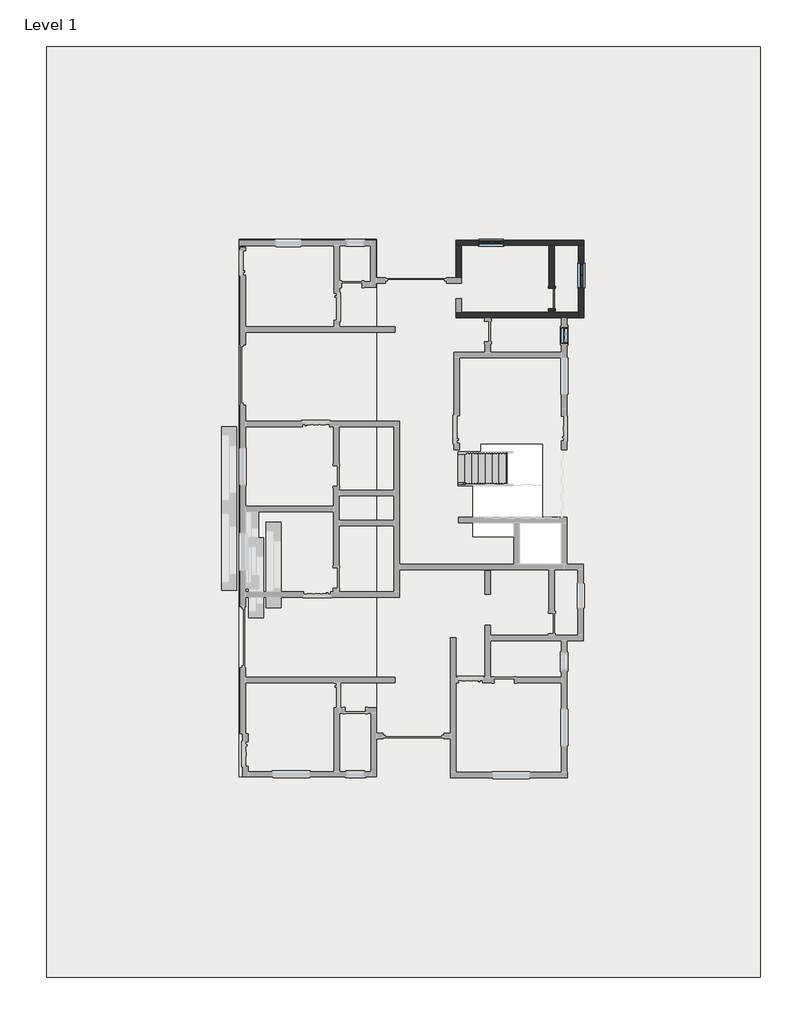
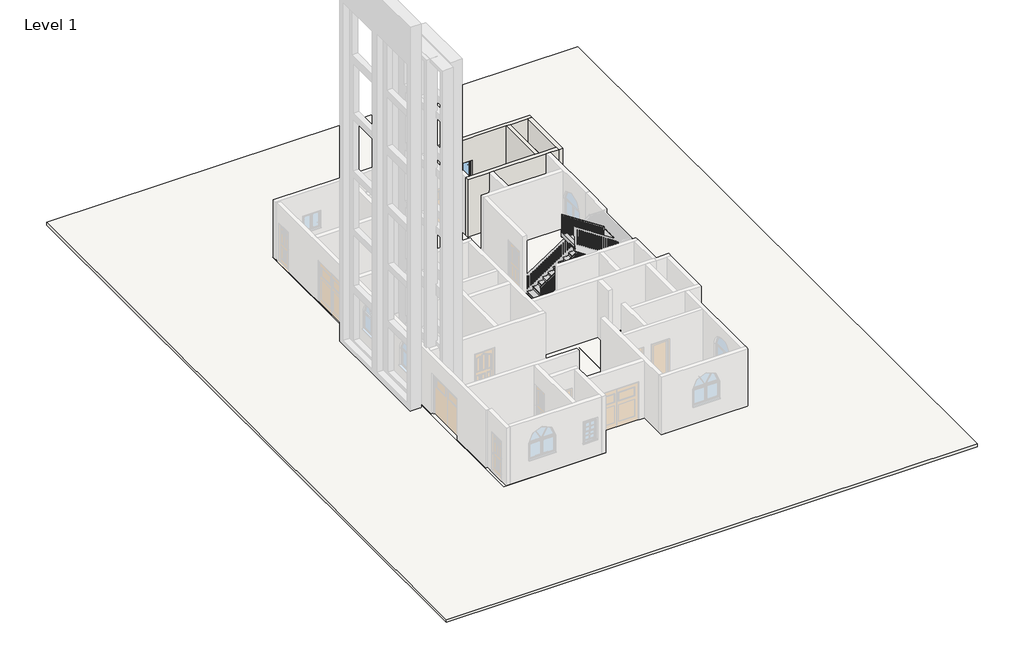
# One storey, part 3 of 4: 5 slabs, 5 walls, 3 windows, 1 door, 1 railing, 1 stair flight.
"""IFC4 building model written with IfcOpenShell, lengths in millimetres."""

from ifc_helpers import new_model, si_unit, frame, origin, origin_with_axes, place, context, project, spatial, polyline, outline, extrude, faceted_brep, transform, mapped, element, save
from components import door_53b1b562, stair_flight_20087966, window_679d2811, windows_dbl_w_glazing_bars_910x910mm_41eba874

model = new_model("IFC4")

# Units and contexts
model_context = context("Model", 3, world=origin())
ifc_project = project(units=[si_unit("LENGTHUNIT", "METRE", prefix="MILLI")], contexts=[model_context])

# Site, building, storey
site = spatial("IfcSite", under=ifc_project)
building = spatial("IfcBuilding", under=site)
storey = spatial("IfcBuildingStorey", under=building, Name="Level 1", Elevation=0.0)

# Door
placement = place(None, origin())
door_shape = door_53b1b562(model_context)
element("IfcDoor", 1, ObjectType="Single-Flush : 30\" x 80\"", at=placement, inside=storey, context=model_context, shape_type="MappedRepresentation", body=[
    mapped(door_shape, transform((5304.3890963, 7217.8962251, 0.0), x_axis=(0.0, 1.0, 0.0), y_axis=(-1.0, 0.0, 0.0), z_axis=(0.0, 0.0, 1.0))),
])

# Railing
element("IfcRailing", 2, ObjectType="Handrail - Rectangular", at=placement, inside=storey, context=model_context, shape_type="SolidModel", body=[
    faceted_brep([(1811.8890963, 347.1962251, 1083.7333333), (1811.8890963, 347.1962251, 1022.8084396), (1811.8890963, 296.3962251, 1022.8084396), (1811.8890963, 296.3962251, 1083.7333333), (4804.8326586, 347.1962251, 3065.2832984), (4855.6326586, 347.1962251, 3037.9917613), (4855.6326586, 296.3962251, 3037.9917613), (4804.8326586, 296.3962251, 3065.2832984), (4804.8326586, 347.1962251, 3115.7333333), (4855.6326586, 347.1962251, 3064.9333333), (4855.6326586, 296.3962251, 3064.9333333), (4804.8326586, 296.3962251, 3115.7333333), (4931.8326586, 347.1962251, 3115.7333333), (4931.8326586, 347.1962251, 3064.9333333), (4881.0326586, 296.3962251, 3064.9333333), (4881.0326586, 296.3962251, 3115.7333333), (4931.8326586, 245.5962251, 3115.7333333), (4881.0326586, 245.5962251, 3115.7333333), (4881.0326586, 194.7962251, 3064.9333333), (4931.8326586, 194.7962251, 3064.9333333)], [[[0, 1, 2, 3]], [[1, 0, 4, 5]], [[2, 1, 5, 6]], [[3, 2, 6, 7]], [[0, 3, 7, 4]], [[5, 4, 8, 9]], [[6, 5, 9, 10]], [[7, 6, 10, 11]], [[4, 7, 11, 8]], [[9, 8, 12, 13]], [[10, 9, 13, 14]], [[11, 10, 14, 15]], [[8, 11, 15, 12]], [[16, 17, 18, 19]], [[13, 12, 16, 19]], [[14, 13, 19, 18]], [[15, 14, 18, 17]], [[12, 15, 17, 16]]]),
    faceted_brep([(4931.8326586, 245.5962251, 3115.7333333), (4931.8326586, 194.7962251, 3064.9333333), (4881.0326586, 194.7962251, 3064.9333333), (4881.0326586, 245.5962251, 3115.7333333), (4931.8326586, 245.5962251, 3251.5487637), (4881.0326586, 245.5962251, 3224.2054325), (4881.0326586, 194.7962251, 3224.2054325), (4931.8326586, 194.7962251, 3251.5487637)], [[[0, 1, 2, 3]], [[4, 5, 6, 7]], [[1, 0, 4, 7]], [[2, 1, 7, 6]], [[3, 2, 6, 5]], [[0, 3, 5, 4]]]),
    faceted_brep([(4931.8326586, 194.7962251, 3251.5487637), (4881.0326586, 194.7962251, 3224.2054325), (4881.0326586, 245.5962251, 3224.2054325), (4931.8326586, 245.5962251, 3251.5487637), (2827.8890963, 194.7962251, 4639.7333333), (2827.8890963, 245.5962251, 4639.7333333), (2827.8890963, 245.5962251, 4578.8720992), (2827.8890963, 194.7962251, 4578.8720992)], [[[0, 1, 2, 3]], [[4, 5, 6, 7]], [[1, 0, 4, 7]], [[2, 1, 7, 6]], [[3, 2, 6, 5]], [[0, 3, 5, 4]]]),
    extrude(outline(polyline([(4541.8779923, 2883.9576586), (4554.4472059, 2864.9076586), (3556.0, 2864.9076586), (3556.0, 2883.9576586), (4541.8779923, 2883.9576586)])), frame((0.0, 210.6712251, 0.0), z_axis=(0.0, 1.0, 0.0), x_axis=(0.0, 0.0, 1.0)), (0.0, 0.0, 1.0), 19.05),
    extrude(outline(polyline([(4474.8421864, 2985.5576586), (4487.4114, 2966.5076586), (3556.0, 2966.5076586), (3556.0, 2985.5576586), (4474.8421864, 2985.5576586)])), frame((0.0, 210.6712251, 0.0), z_axis=(0.0, 1.0, 0.0), x_axis=(0.0, 0.0, 1.0)), (0.0, 0.0, 1.0), 19.05),
    extrude(outline(polyline([(4407.8063805, 3087.1576586), (4420.3755941, 3068.1076586), (3556.0, 3068.1076586), (3556.0, 3087.1576586), (4407.8063805, 3087.1576586)])), frame((0.0, 210.6712251, 0.0), z_axis=(0.0, 1.0, 0.0), x_axis=(0.0, 0.0, 1.0)), (0.0, 0.0, 1.0), 19.05),
    extrude(outline(polyline([(4340.7705746, 3188.7576586), (4353.3397882, 3169.7076586), (3386.6666667, 3169.7076586), (3386.6666667, 3188.7576586), (4340.7705746, 3188.7576586)])), frame((0.0, 210.6712251, 0.0), z_axis=(0.0, 1.0, 0.0), x_axis=(0.0, 0.0, 1.0)), (0.0, 0.0, 1.0), 19.05),
    extrude(outline(polyline([(4273.7347687, 3290.3576586), (4286.3039823, 3271.3076586), (3386.6666667, 3271.3076586), (3386.6666667, 3290.3576586), (4273.7347687, 3290.3576586)])), frame((0.0, 210.6712251, 0.0), z_axis=(0.0, 1.0, 0.0), x_axis=(0.0, 0.0, 1.0)), (0.0, 0.0, 1.0), 19.05),
    extrude(outline(polyline([(4206.6989628, 3391.9576586), (4219.2681764, 3372.9076586), (3217.3333333, 3372.9076586), (3217.3333333, 3391.9576586), (4206.6989628, 3391.9576586)])), frame((0.0, 210.6712251, 0.0), z_axis=(0.0, 1.0, 0.0), x_axis=(0.0, 0.0, 1.0)), (0.0, 0.0, 1.0), 19.05),
    extrude(outline(polyline([(4139.6631569, 3493.5576586), (4152.2323705, 3474.5076586), (3217.3333333, 3474.5076586), (3217.3333333, 3493.5576586), (4139.6631569, 3493.5576586)])), frame((0.0, 210.6712251, 0.0), z_axis=(0.0, 1.0, 0.0), x_axis=(0.0, 0.0, 1.0)), (0.0, 0.0, 1.0), 19.05),
    extrude(outline(polyline([(4072.627351, 3595.1576586), (4085.1965646, 3576.1076586), (3217.3333333, 3576.1076586), (3217.3333333, 3595.1576586), (4072.627351, 3595.1576586)])), frame((0.0, 210.6712251, 0.0), z_axis=(0.0, 1.0, 0.0), x_axis=(0.0, 0.0, 1.0)), (0.0, 0.0, 1.0), 19.05),
    extrude(outline(polyline([(4005.5915451, 3696.7576586), (4018.1607587, 3677.7076586), (3048.0, 3677.7076586), (3048.0, 3696.7576586), (4005.5915451, 3696.7576586)])), frame((0.0, 210.6712251, 0.0), z_axis=(0.0, 1.0, 0.0), x_axis=(0.0, 0.0, 1.0)), (0.0, 0.0, 1.0), 19.05),
    extrude(outline(polyline([(3938.5557392, 3798.3576586), (3951.1249528, 3779.3076586), (3048.0, 3779.3076586), (3048.0, 3798.3576586), (3938.5557392, 3798.3576586)])), frame((0.0, 210.6712251, 0.0), z_axis=(0.0, 1.0, 0.0), x_axis=(0.0, 0.0, 1.0)), (0.0, 0.0, 1.0), 19.05),
    extrude(outline(polyline([(3871.5199333, 3899.9576586), (3884.0891469, 3880.9076586), (2878.6666667, 3880.9076586), (2878.6666667, 3899.9576586), (3871.5199333, 3899.9576586)])), frame((0.0, 210.6712251, 0.0), z_axis=(0.0, 1.0, 0.0), x_axis=(0.0, 0.0, 1.0)), (0.0, 0.0, 1.0), 19.05),
    extrude(outline(polyline([(3804.4841274, 4001.5576586), (3817.053341, 3982.5076586), (2878.6666667, 3982.5076586), (2878.6666667, 4001.5576586), (3804.4841274, 4001.5576586)])), frame((0.0, 210.6712251, 0.0), z_axis=(0.0, 1.0, 0.0), x_axis=(0.0, 0.0, 1.0)), (0.0, 0.0, 1.0), 19.05),
    extrude(outline(polyline([(3737.4483215, 4103.1576586), (3750.0175351, 4084.1076586), (2878.6666667, 4084.1076586), (2878.6666667, 4103.1576586), (3737.4483215, 4103.1576586)])), frame((0.0, 210.6712251, 0.0), z_axis=(0.0, 1.0, 0.0), x_axis=(0.0, 0.0, 1.0)), (0.0, 0.0, 1.0), 19.05),
    extrude(outline(polyline([(3670.4125156, 4204.7576586), (3682.9817292, 4185.7076586), (2709.3333333, 4185.7076586), (2709.3333333, 4204.7576586), (3670.4125156, 4204.7576586)])), frame((0.0, 210.6712251, 0.0), z_axis=(0.0, 1.0, 0.0), x_axis=(0.0, 0.0, 1.0)), (0.0, 0.0, 1.0), 19.05),
    extrude(outline(polyline([(3603.3767097, 4306.3576586), (3615.9459233, 4287.3076586), (2709.3333333, 4287.3076586), (2709.3333333, 4306.3576586), (3603.3767097, 4306.3576586)])), frame((0.0, 210.6712251, 0.0), z_axis=(0.0, 1.0, 0.0), x_axis=(0.0, 0.0, 1.0)), (0.0, 0.0, 1.0), 19.05),
    extrude(outline(polyline([(3536.3409038, 4407.9576586), (3548.9101174, 4388.9076586), (2540.0, 4388.9076586), (2540.0, 4407.9576586), (3536.3409038, 4407.9576586)])), frame((0.0, 210.6712251, 0.0), z_axis=(0.0, 1.0, 0.0), x_axis=(0.0, 0.0, 1.0)), (0.0, 0.0, 1.0), 19.05),
    extrude(outline(polyline([(3469.3050979, 4509.5576586), (3481.8743115, 4490.5076586), (2540.0, 4490.5076586), (2540.0, 4509.5576586), (3469.3050979, 4509.5576586)])), frame((0.0, 210.6712251, 0.0), z_axis=(0.0, 1.0, 0.0), x_axis=(0.0, 0.0, 1.0)), (0.0, 0.0, 1.0), 19.05),
    extrude(outline(polyline([(3402.269292, 4611.1576586), (3414.8385056, 4592.1076586), (2540.0, 4592.1076586), (2540.0, 4611.1576586), (3402.269292, 4611.1576586)])), frame((0.0, 210.6712251, 0.0), z_axis=(0.0, 1.0, 0.0), x_axis=(0.0, 0.0, 1.0)), (0.0, 0.0, 1.0), 19.05),
    extrude(outline(polyline([(3335.2334861, 4712.7576586), (3347.8026997, 4693.7076586), (2370.6666667, 4693.7076586), (2370.6666667, 4712.7576586), (3335.2334861, 4712.7576586)])), frame((0.0, 210.6712251, 0.0), z_axis=(0.0, 1.0, 0.0), x_axis=(0.0, 0.0, 1.0)), (0.0, 0.0, 1.0), 19.05),
    extrude(outline(polyline([(3268.1976802, 4814.3576586), (3280.7668938, 4795.3076586), (2370.6666667, 4795.3076586), (2370.6666667, 4814.3576586), (3268.1976802, 4814.3576586)])), frame((0.0, 210.6712251, 0.0), z_axis=(0.0, 1.0, 0.0), x_axis=(0.0, 0.0, 1.0)), (0.0, 0.0, 1.0), 19.05),
    extrude(outline(polyline([(4850.3640963, 312.2712251), (4850.3640963, 331.3212251), (4869.4140963, 331.3212251), (4869.4140963, 312.2712251), (4850.3640963, 312.2712251)])), frame((0.0, 0.0, 2032.0), z_axis=(0.0, 0.0, 1.0), x_axis=(1.0, 0.0, 0.0)), (0.0, 0.0, 1.0), 1032.9333333),
    extrude(outline(polyline([(2979.8493789, 4767.8140963), (2967.2368701, 4748.7640963), (2032.0, 4748.7640963), (2032.0, 4767.8140963), (2979.8493789, 4767.8140963)])), frame((0.0, 312.2712251, 0.0), z_axis=(0.0, 1.0, 0.0), x_axis=(0.0, 0.0, 1.0)), (0.0, 0.0, 1.0), 19.05),
    extrude(outline(polyline([(2912.5826656, 4666.2140963), (2899.9701569, 4647.1640963), (2032.0, 4647.1640963), (2032.0, 4666.2140963), (2912.5826656, 4666.2140963)])), frame((0.0, 312.2712251, 0.0), z_axis=(0.0, 1.0, 0.0), x_axis=(0.0, 0.0, 1.0)), (0.0, 0.0, 1.0), 19.05),
    extrude(outline(polyline([(2845.3159523, 4564.6140963), (2832.7034436, 4545.5640963), (1862.6666667, 4545.5640963), (1862.6666667, 4564.6140963), (2845.3159523, 4564.6140963)])), frame((0.0, 312.2712251, 0.0), z_axis=(0.0, 1.0, 0.0), x_axis=(0.0, 0.0, 1.0)), (0.0, 0.0, 1.0), 19.05),
    extrude(outline(polyline([(2778.049239, 4463.0140963), (2765.4367303, 4443.9640963), (1862.6666667, 4443.9640963), (1862.6666667, 4463.0140963), (2778.049239, 4463.0140963)])), frame((0.0, 312.2712251, 0.0), z_axis=(0.0, 1.0, 0.0), x_axis=(0.0, 0.0, 1.0)), (0.0, 0.0, 1.0), 19.05),
    extrude(outline(polyline([(2710.7825258, 4361.4140963), (2698.170017, 4342.3640963), (1862.6666667, 4342.3640963), (1862.6666667, 4361.4140963), (2710.7825258, 4361.4140963)])), frame((0.0, 312.2712251, 0.0), z_axis=(0.0, 1.0, 0.0), x_axis=(0.0, 0.0, 1.0)), (0.0, 0.0, 1.0), 19.05),
    extrude(outline(polyline([(2643.5158125, 4259.8140963), (2630.9033038, 4240.7640963), (1693.3333333, 4240.7640963), (1693.3333333, 4259.8140963), (2643.5158125, 4259.8140963)])), frame((0.0, 312.2712251, 0.0), z_axis=(0.0, 1.0, 0.0), x_axis=(0.0, 0.0, 1.0)), (0.0, 0.0, 1.0), 19.05),
    extrude(outline(polyline([(2576.2490992, 4158.2140963), (2563.6365905, 4139.1640963), (1693.3333333, 4139.1640963), (1693.3333333, 4158.2140963), (2576.2490992, 4158.2140963)])), frame((0.0, 312.2712251, 0.0), z_axis=(0.0, 1.0, 0.0), x_axis=(0.0, 0.0, 1.0)), (0.0, 0.0, 1.0), 19.05),
    extrude(outline(polyline([(2508.982386, 4056.6140963), (2496.3698772, 4037.5640963), (1524.0, 4037.5640963), (1524.0, 4056.6140963), (2508.982386, 4056.6140963)])), frame((0.0, 312.2712251, 0.0), z_axis=(0.0, 1.0, 0.0), x_axis=(0.0, 0.0, 1.0)), (0.0, 0.0, 1.0), 19.05),
    extrude(outline(polyline([(2441.7156727, 3955.0140963), (2429.1031639, 3935.9640963), (1524.0, 3935.9640963), (1524.0, 3955.0140963), (2441.7156727, 3955.0140963)])), frame((0.0, 312.2712251, 0.0), z_axis=(0.0, 1.0, 0.0), x_axis=(0.0, 0.0, 1.0)), (0.0, 0.0, 1.0), 19.05),
    extrude(outline(polyline([(2374.4489594, 3853.4140963), (2361.8364507, 3834.3640963), (1524.0, 3834.3640963), (1524.0, 3853.4140963), (2374.4489594, 3853.4140963)])), frame((0.0, 312.2712251, 0.0), z_axis=(0.0, 1.0, 0.0), x_axis=(0.0, 0.0, 1.0)), (0.0, 0.0, 1.0), 19.05),
    extrude(outline(polyline([(2307.1822461, 3751.8140963), (2294.5697374, 3732.7640963), (1354.6666667, 3732.7640963), (1354.6666667, 3751.8140963), (2307.1822461, 3751.8140963)])), frame((0.0, 312.2712251, 0.0), z_axis=(0.0, 1.0, 0.0), x_axis=(0.0, 0.0, 1.0)), (0.0, 0.0, 1.0), 19.05),
    extrude(outline(polyline([(2239.9155329, 3650.2140963), (2227.3030241, 3631.1640963), (1354.6666667, 3631.1640963), (1354.6666667, 3650.2140963), (2239.9155329, 3650.2140963)])), frame((0.0, 312.2712251, 0.0), z_axis=(0.0, 1.0, 0.0), x_axis=(0.0, 0.0, 1.0)), (0.0, 0.0, 1.0), 19.05),
    extrude(outline(polyline([(2172.6488196, 3548.6140963), (2160.0363109, 3529.5640963), (1185.3333333, 3529.5640963), (1185.3333333, 3548.6140963), (2172.6488196, 3548.6140963)])), frame((0.0, 312.2712251, 0.0), z_axis=(0.0, 1.0, 0.0), x_axis=(0.0, 0.0, 1.0)), (0.0, 0.0, 1.0), 19.05),
    extrude(outline(polyline([(2105.3821063, 3447.0140963), (2092.7695976, 3427.9640963), (1185.3333333, 3427.9640963), (1185.3333333, 3447.0140963), (2105.3821063, 3447.0140963)])), frame((0.0, 312.2712251, 0.0), z_axis=(0.0, 1.0, 0.0), x_axis=(0.0, 0.0, 1.0)), (0.0, 0.0, 1.0), 19.05),
    extrude(outline(polyline([(2038.115393, 3345.4140963), (2025.5028843, 3326.3640963), (1185.3333333, 3326.3640963), (1185.3333333, 3345.4140963), (2038.115393, 3345.4140963)])), frame((0.0, 312.2712251, 0.0), z_axis=(0.0, 1.0, 0.0), x_axis=(0.0, 0.0, 1.0)), (0.0, 0.0, 1.0), 19.05),
    extrude(outline(polyline([(1970.8486798, 3243.8140963), (1958.236171, 3224.7640963), (1016.0, 3224.7640963), (1016.0, 3243.8140963), (1970.8486798, 3243.8140963)])), frame((0.0, 312.2712251, 0.0), z_axis=(0.0, 1.0, 0.0), x_axis=(0.0, 0.0, 1.0)), (0.0, 0.0, 1.0), 19.05),
    extrude(outline(polyline([(1903.5819665, 3142.2140963), (1890.9694578, 3123.1640963), (1016.0, 3123.1640963), (1016.0, 3142.2140963), (1903.5819665, 3142.2140963)])), frame((0.0, 312.2712251, 0.0), z_axis=(0.0, 1.0, 0.0), x_axis=(0.0, 0.0, 1.0)), (0.0, 0.0, 1.0), 19.05),
    extrude(outline(polyline([(1836.3152532, 3040.6140963), (1823.7027445, 3021.5640963), (846.6666667, 3021.5640963), (846.6666667, 3040.6140963), (1836.3152532, 3040.6140963)])), frame((0.0, 312.2712251, 0.0), z_axis=(0.0, 1.0, 0.0), x_axis=(0.0, 0.0, 1.0)), (0.0, 0.0, 1.0), 19.05),
    extrude(outline(polyline([(1769.04854, 2939.0140963), (1756.4360312, 2919.9640963), (846.6666667, 2919.9640963), (846.6666667, 2939.0140963), (1769.04854, 2939.0140963)])), frame((0.0, 312.2712251, 0.0), z_axis=(0.0, 1.0, 0.0), x_axis=(0.0, 0.0, 1.0)), (0.0, 0.0, 1.0), 19.05),
    extrude(outline(polyline([(1701.7818267, 2837.4140963), (1689.1693179, 2818.3640963), (846.6666667, 2818.3640963), (846.6666667, 2837.4140963), (1701.7818267, 2837.4140963)])), frame((0.0, 312.2712251, 0.0), z_axis=(0.0, 1.0, 0.0), x_axis=(0.0, 0.0, 1.0)), (0.0, 0.0, 1.0), 19.05),
    extrude(outline(polyline([(1634.5151134, 2735.8140963), (1621.9026047, 2716.7640963), (677.3333333, 2716.7640963), (677.3333333, 2735.8140963), (1634.5151134, 2735.8140963)])), frame((0.0, 312.2712251, 0.0), z_axis=(0.0, 1.0, 0.0), x_axis=(0.0, 0.0, 1.0)), (0.0, 0.0, 1.0), 19.05),
    extrude(outline(polyline([(1567.2484001, 2634.2140963), (1554.6358914, 2615.1640963), (677.3333333, 2615.1640963), (677.3333333, 2634.2140963), (1567.2484001, 2634.2140963)])), frame((0.0, 312.2712251, 0.0), z_axis=(0.0, 1.0, 0.0), x_axis=(0.0, 0.0, 1.0)), (0.0, 0.0, 1.0), 19.05),
    extrude(outline(polyline([(1499.9816869, 2532.6140963), (1487.3691781, 2513.5640963), (508.0, 2513.5640963), (508.0, 2532.6140963), (1499.9816869, 2532.6140963)])), frame((0.0, 312.2712251, 0.0), z_axis=(0.0, 1.0, 0.0), x_axis=(0.0, 0.0, 1.0)), (0.0, 0.0, 1.0), 19.05),
    extrude(outline(polyline([(1432.7149736, 2431.0140963), (1420.1024649, 2411.9640963), (508.0, 2411.9640963), (508.0, 2431.0140963), (1432.7149736, 2431.0140963)])), frame((0.0, 312.2712251, 0.0), z_axis=(0.0, 1.0, 0.0), x_axis=(0.0, 0.0, 1.0)), (0.0, 0.0, 1.0), 19.05),
    extrude(outline(polyline([(1365.4482603, 2329.4140963), (1352.8357516, 2310.3640963), (508.0, 2310.3640963), (508.0, 2329.4140963), (1365.4482603, 2329.4140963)])), frame((0.0, 312.2712251, 0.0), z_axis=(0.0, 1.0, 0.0), x_axis=(0.0, 0.0, 1.0)), (0.0, 0.0, 1.0), 19.05),
    extrude(outline(polyline([(1298.181547, 2227.8140963), (1285.5690383, 2208.7640963), (338.6666667, 2208.7640963), (338.6666667, 2227.8140963), (1298.181547, 2227.8140963)])), frame((0.0, 312.2712251, 0.0), z_axis=(0.0, 1.0, 0.0), x_axis=(0.0, 0.0, 1.0)), (0.0, 0.0, 1.0), 19.05),
    extrude(outline(polyline([(1230.9148338, 2126.2140963), (1218.302325, 2107.1640963), (338.6666667, 2107.1640963), (338.6666667, 2126.2140963), (1230.9148338, 2126.2140963)])), frame((0.0, 312.2712251, 0.0), z_axis=(0.0, 1.0, 0.0), x_axis=(0.0, 0.0, 1.0)), (0.0, 0.0, 1.0), 19.05),
    extrude(outline(polyline([(1163.6481205, 2024.6140963), (1151.0356118, 2005.5640963), (169.3333333, 2005.5640963), (169.3333333, 2024.6140963), (1163.6481205, 2024.6140963)])), frame((0.0, 312.2712251, 0.0), z_axis=(0.0, 1.0, 0.0), x_axis=(0.0, 0.0, 1.0)), (0.0, 0.0, 1.0), 19.05),
    extrude(outline(polyline([(1096.3814072, 1923.0140963), (1083.7688985, 1903.9640963), (169.3333333, 1903.9640963), (169.3333333, 1923.0140963), (1096.3814072, 1923.0140963)])), frame((0.0, 312.2712251, 0.0), z_axis=(0.0, 1.0, 0.0), x_axis=(0.0, 0.0, 1.0)), (0.0, 0.0, 1.0), 19.05),
    extrude(outline(polyline([(4896.9076586, 229.7212251), (4915.9576586, 229.7212251), (4915.9576586, 210.6712251), (4896.9076586, 210.6712251), (4896.9076586, 229.7212251)])), frame((0.0, 0.0, 2201.3333333), z_axis=(0.0, 0.0, 1.0), x_axis=(1.0, 0.0, 0.0)), (0.0, 0.0, 1.0), 863.6),
    extrude(outline(polyline([(4896.9076586, 312.2712251), (4896.9076586, 331.3212251), (4915.9576586, 331.3212251), (4915.9576586, 312.2712251), (4896.9076586, 312.2712251)])), frame((0.0, 0.0, 2201.3333333), z_axis=(0.0, 0.0, 1.0), x_axis=(1.0, 0.0, 0.0)), (0.0, 0.0, 1.0), 863.6),
    extrude(outline(polyline([(4566.3028856, 2846.9390963), (4578.8720992, 2827.8890963), (3556.0, 2827.8890963), (3556.0, 2846.9390963), (4566.3028856, 2846.9390963)])), frame((0.0, 210.6712251, 0.0), z_axis=(0.0, 1.0, 0.0), x_axis=(0.0, 0.0, 1.0)), (0.0, 0.0, 1.0), 19.05),
    extrude(outline(polyline([(1035.4209483, 1830.9390963), (1022.8084396, 1811.8890963), (169.3333333, 1811.8890963), (169.3333333, 1830.9390963), (1035.4209483, 1830.9390963)])), frame((0.0, 312.2712251, 0.0), z_axis=(0.0, 1.0, 0.0), x_axis=(0.0, 0.0, 1.0)), (0.0, 0.0, 1.0), 19.05),
])

# Slabs
element("IfcSlab", 3, ObjectType="Generic - 12\"", at=placement, inside=storey, context=model_context, shape_type="SweptSolid", body=[
    extrude(outline(polyline([(5875.8890963, 9402.2962251), (5875.8890963, -10638.3037749), (1722.9890963, -10638.3037749), (1722.9890963, 9402.2962251), (5875.8890963, 9402.2962251)]), holes=[polyline([(4097.8890963, -2688.1037749), (5659.9890963, -2688.1037749), (5659.9890963, -1138.7037749), (4791.2853127, -1138.7037749), (4791.2853127, -958.5315685), (4949.8616623, -958.5315685), (4949.8616623, 1784.6684315), (2663.8616623, 1784.6684315), (2663.8616623, 941.43649), (2352.8853127, 941.43649), (2352.8853127, -1649.36351), (4097.8890963, -1649.36351), (4097.8890963, -2688.1037749)])]), frame((0.0, 0.0, -152.4), z_axis=(0.0, 0.0, 1.0), x_axis=(1.0, 0.0, 0.0)), (0.0, 0.0, 1.0), 152.4),
])
element("IfcSlab", 4, ObjectType="Generic - 12\"", at=placement, inside=storey, context=model_context, shape_type="SweptSolid", body=[
    extrude(outline(polyline([(6498.1890963, 9402.2962251), (6498.1890963, 6506.6962251), (5875.8890963, 6506.6962251), (5875.8890963, 9402.2962251), (6498.1890963, 9402.2962251)])), frame((0.0, 0.0, -152.4), z_axis=(0.0, 0.0, 1.0), x_axis=(1.0, 0.0, 0.0)), (0.0, 0.0, 1.0), 152.4),
])
element("IfcSlab", 5, ObjectType="Generic - 12\"", at=placement, inside=storey, context=model_context, shape_type="SweptSolid", body=[
    extrude(outline(polyline([(6485.4890963, -2688.1037749), (6485.4890963, -5532.9037749), (5863.1890963, -5532.9037749), (5863.1890963, -2688.1037749), (6485.4890963, -2688.1037749)])), frame((0.0, 0.0, -152.4), z_axis=(0.0, 0.0, 1.0), x_axis=(1.0, 0.0, 0.0)), (0.0, 0.0, 1.0), 152.4),
])
element("IfcSlab", 6, ObjectType="Generic - 12\"", at=placement, inside=storey, context=model_context, shape_type="SweptSolid", body=[
    extrude(outline(polyline([(-1236.1109037, 9427.2527313), (-1236.1109037, -10612.9037749), (-6354.2109037, -10612.9037749), (-6354.2109037, 9427.2527313), (-1236.1109037, 9427.2527313)])), frame((0.0, 0.0, -152.4), z_axis=(0.0, 0.0, 1.0), x_axis=(1.0, 0.0, 0.0)), (0.0, 0.0, 1.0), 152.4),
])
element("IfcSlab", 7, ObjectType="Generic - 12\"", at=placement, inside=storey, context=model_context, shape_type="SweptSolid", body=[
    extrude(outline(polyline([(13076.7890963, 16615.4527313), (13076.7890963, -18086.1761038), (-13544.4013636, -18086.1761038), (-13544.4013636, 16615.4527313), (13076.7890963, 16615.4527313)]), holes=[polyline([(4097.8890963, -2688.1037749), (5659.9890963, -2688.1037749), (5659.9890963, -1138.7037749), (4791.2853127, -1138.7037749), (4791.2853127, -958.5315685), (4949.8616623, -958.5315685), (4949.8616623, 1784.6684315), (2663.8616623, 1784.6684315), (2663.8616623, 941.43649), (2352.8853127, 941.43649), (2352.8853127, -1649.36351), (4097.8890963, -1649.36351), (4097.8890963, -2688.1037749)])]), frame((0.0, 0.0, -152.4), z_axis=(0.0, 0.0, 1.0), x_axis=(1.0, 0.0, 0.0)), (0.0, 0.0, 1.0), 152.4),
])

# Stair flight
stair_flight_shape = stair_flight_20087966(model_context)
element("IfcStairFlight", 8, ObjectType="2\" Tread 1\" Nosing 1/4\" Riser", at=placement, inside=storey, context=model_context, shape_type="MappedRepresentation", body=[
    mapped(stair_flight_shape, transform((0.0, 0.0, 0.0), x_axis=(1.0, 0.0, 0.0), y_axis=(0.0, 1.0, 0.0), z_axis=(0.0, 0.0, 1.0))),
])

# Walls
element("IfcWall", 9, ObjectType="Generic - 9\" w", at=placement, inside=storey, context=model_context, shape_type="Brep", body=[
    faceted_brep([(1722.9890963, 9199.0962251, 0.0), (1926.1890963, 9199.0962251, 0.0), (5202.7890963, 9199.0962251, 0.0), (5405.9890963, 9199.0962251, 0.0), (6294.9890963, 9199.0962251, 0.0), (6498.1890963, 9199.0962251, 0.0), (6498.1890963, 9199.0962251, 3048.0), (6294.9890963, 9199.0962251, 3048.0), (5405.9890963, 9199.0962251, 3048.0), (5202.7890963, 9199.0962251, 3048.0), (1926.1890963, 9199.0962251, 3048.0), (1722.9890963, 9199.0962251, 3048.0), (2588.7890963, 9199.0962251, 1824.4), (3498.7890963, 9199.0962251, 1824.4), (3498.7890963, 9199.0962251, 914.4), (2588.7890963, 9199.0962251, 914.4), (1722.9890963, 9402.2962251, 0.0), (1722.9890963, 9402.2962251, 3048.0), (6498.1890963, 9402.2962251, 3048.0), (6498.1890963, 9402.2962251, 0.0), (2588.7890963, 9402.2962251, 1824.4), (2588.7890963, 9402.2962251, 914.4), (3498.7890963, 9402.2962251, 914.4), (3498.7890963, 9402.2962251, 1824.4)], [[[0, 1, 2, 3, 4, 5, 6, 7, 8, 9, 10, 11], [12, 13, 14, 15]], [[16, 17, 18, 19], [20, 21, 22, 23]], [[5, 4, 3, 2, 1, 0, 16, 19]], [[11, 10, 9, 8, 7, 6, 18, 17]], [[0, 11, 17, 16]], [[6, 5, 19, 18]], [[21, 20, 12, 15]], [[22, 21, 15, 14]], [[23, 22, 14, 13]], [[20, 23, 13, 12]]]),
])
element("IfcWall", 10, ObjectType="Generic -4.5\" p", at=placement, inside=storey, context=model_context, shape_type="SweptSolid", body=[
    extrude(outline(polyline([(1722.9890963, 7992.5962251), (1722.9890963, 9199.0962251), (1926.1890963, 9199.0962251), (1926.1890963, 7992.5962251), (1722.9890963, 7992.5962251)])), origin_with_axes(), (0.0, 0.0, 1.0), 3048.0),
])
element("IfcWall", 11, ObjectType="Generic -4.5\" p", at=placement, inside=storey, context=model_context, shape_type="SweptSolid", body=[
    extrude(outline(polyline([(9199.0962251, 0.0), (7598.8962251, 0.0), (7598.8962251, 2032.0), (6836.8962251, 2032.0), (6836.8962251, 0.0), (6709.8962251, 0.0), (6709.8962251, 3048.0), (9199.0962251, 3048.0), (9199.0962251, 0.0)])), frame((5202.7890963, 0.0, 0.0), z_axis=(1.0, 0.0, 0.0), x_axis=(0.0, 1.0, 0.0)), (0.0, 0.0, 1.0), 203.2),
])
element("IfcWall", 12, ObjectType="Generic -4.5\" p", at=placement, inside=storey, context=model_context, shape_type="Brep", body=[
    faceted_brep([(6294.9890963, 9199.0962251, 0.0), (6294.9890963, 6709.8962251, 0.0), (6294.9890963, 6506.6962251, 0.0), (6294.9890963, 6506.6962251, 3048.0), (6294.9890963, 6709.8962251, 3048.0), (6294.9890963, 9199.0962251, 3048.0), (6294.9890963, 8536.4962251, 1824.4), (6294.9890963, 7626.4962251, 1824.4), (6294.9890963, 7626.4962251, 914.4), (6294.9890963, 8536.4962251, 914.4), (6498.1890963, 9199.0962251, 0.0), (6498.1890963, 9199.0962251, 3048.0), (6498.1890963, 6506.6962251, 3048.0), (6498.1890963, 6506.6962251, 0.0), (6498.1890963, 8536.4962251, 1824.4), (6498.1890963, 8536.4962251, 914.4), (6498.1890963, 7626.4962251, 914.4), (6498.1890963, 7626.4962251, 1824.4)], [[[0, 1, 2, 3, 4, 5], [6, 7, 8, 9]], [[10, 11, 12, 13], [14, 15, 16, 17]], [[2, 1, 0, 10, 13]], [[5, 4, 3, 12, 11]], [[3, 2, 13, 12]], [[0, 5, 11, 10]], [[15, 14, 6, 9]], [[16, 15, 9, 8]], [[17, 16, 8, 7]], [[14, 17, 7, 6]]]),
])
element("IfcWall", 13, ObjectType="Generic -4.5\" p", at=placement, inside=storey, context=model_context, shape_type="Brep", body=[
    faceted_brep([(6294.9890963, 6709.8962251, 0.0), (5405.9890963, 6709.8962251, 0.0), (5202.7890963, 6709.8962251, 0.0), (1926.1890963, 6709.8962251, 0.0), (1722.9890963, 6709.8962251, 0.0), (1722.9890963, 6709.8962251, 3048.0), (1926.1890963, 6709.8962251, 3048.0), (5202.7890963, 6709.8962251, 3048.0), (5405.9890963, 6709.8962251, 3048.0), (6294.9890963, 6709.8962251, 3048.0), (6294.9890963, 6506.6962251, 0.0), (6294.9890963, 6506.6962251, 3048.0), (5863.1890963, 6506.6962251, 3048.0), (5659.9890963, 6506.6962251, 3048.0), (3018.3890963, 6506.6962251, 3048.0), (2815.1890963, 6506.6962251, 3048.0), (1722.9890963, 6506.6962251, 3048.0), (1722.9890963, 6506.6962251, 0.0), (2815.1890963, 6506.6962251, 0.0), (3018.3890963, 6506.6962251, 0.0), (5659.9890963, 6506.6962251, 0.0), (5863.1890963, 6506.6962251, 0.0)], [[[0, 1, 2, 3, 4, 5, 6, 7, 8, 9]], [[10, 11, 12, 13, 14, 15, 16, 17, 18, 19, 20, 21]], [[4, 3, 2, 1, 0, 10, 21, 20, 19, 18, 17]], [[9, 8, 7, 6, 5, 16, 15, 14, 13, 12, 11]], [[0, 9, 11, 10]], [[5, 4, 17, 16]]]),
])

# Windows
window_shape = window_679d2811(model_context)
element("IfcWindow", 14, ObjectType="Window-Double-Hung : 24\" x 42\"", at=placement, inside=storey, context=model_context, shape_type="MappedRepresentation", body=[
    mapped(window_shape, transform((5761.5890963, 5846.2962251, 0.0), x_axis=(0.0, -1.0, 0.0), y_axis=(1.0, 0.0, 0.0), z_axis=(0.0, 0.0, 1.0))),
])
windows_dbl_w_glazing_bars_910x910mm_shape = windows_dbl_w_glazing_bars_910x910mm_41eba874(model_context)
element("IfcWindow", 15, ObjectType="Windows_Dbl_w-Glazing_Bars : 910x910mm", at=placement, inside=storey, context=model_context, shape_type="MappedRepresentation", body=[
    mapped(windows_dbl_w_glazing_bars_910x910mm_shape, transform((6388.1325284, 7951.4962251, -275.6), x_axis=(0.0, -1.0, 0.0), y_axis=(1.0, 0.0, 0.0), z_axis=(0.0, 0.0, 1.0))),
])
element("IfcWindow", 16, ObjectType="Windows_Dbl_w-Glazing_Bars : 910x910mm", at=placement, inside=storey, context=model_context, shape_type="MappedRepresentation", body=[
    mapped(windows_dbl_w_glazing_bars_910x910mm_shape, transform((3173.7890963, 9292.2396573, -275.6), x_axis=(1.0, 0.0, 0.0), y_axis=(0.0, 1.0, 0.0), z_axis=(0.0, 0.0, 1.0))),
])

save(model, "model.ifc")

# Revit data of these elements
# Type "Single-Flush : 30\" x 80\""
#   Type Mark = "5"
#   Construction Type Id = "MDOOR"
#   Assembly Code = "C1020"
#   Analytic Construction = "Metal"
#   Thickness = 0' - 2"
#   Heat Transfer Coefficient (U) = 0.651978 BTU/(h·ft²·°F)
#   Height = 6' - 8"
#   Trim Projection Ext = 0' - 1"
#   Trim Projection Int = 0' - 1"
#   Trim Width = 0' - 3"
#   Width = 2' - 6"
#   Define Thermal Properties by = 1
#   Define Thermal Properties by = 1
#   Door Material = Door - Panel
#   Frame Material = Door - Frame
#   Visual Light Transmittance = 0
#   Solar Heat Gain Coefficient = 0
#   Function = (empty or 0)
#   Wall Closure = (empty or 0)
# Type "Handrail - Rectangular"
#   Assembly Code = "C2010400"
#   built-in parameter 1008612 = 0.0416667 (stored number, unit not read)
#   built-in parameter 1008611 = 0.0416667 (stored number, unit not read)
#   built-in parameter 1008609 = 0.333333 (stored number, unit not read)
#   built-in parameter 1008604 = 0.166667 (stored number, unit not read)
#   built-in parameter 1008603 = 0.166667 (stored number, unit not read)
#   Railing Height = 3' - 0"
#   built-in parameter 1008630 = 2
#   built-in parameter 1008610 = 2
#   built-in parameter 1008618 = Baluster - Square : 3/4"
# Type "Generic - 12\""
#   Assembly Code = "B1010"
#   Function = 0
#   Layers, outside or top first: 0' - 6" no material (function 1)
# Type "Generic - 9\" w"
#   Assembly Code = "B2010"
#   Layers, outside or top first: 0' - 8" no material (function 1)
# Type "Generic -4.5\" p"
#   Assembly Code = "B2010"
#   Layers, outside or top first: 0' - 8" no material (function 1)
# Type "Window-Double-Hung : 24\" x 42\""
#   Type Mark = "10"
#   Fire Rating = "0.5h"
#   Construction Type Id = "DG-DR"
#   Assembly Code = "B2020100"
#   Analytic Construction = "Double glazing - domestic"
#   Wall Thickness [instance default] = 0' - 6"
#   Window Inset [instance default] = 0' - 0"
#   Visual Light Transmittance = 0.81
#   Thermal Resistance (R) = 1.8146 (h·ft²·°F)/BTU
#   Solar Heat Gain Coefficient = 0.76
#   Muntin Width = 1' - 6"
#   Muntin Height = 1' - 5 1/8"
#   Interior Wall Closure [instance default] = 0' - 1 1/2"
#   Rough Width = 2' - 0 1/2"
#   Rough Height = 3' - 6 1/2"
#   Frame Extension [instance default] = 0' - 1 1/4"
#   Exterior Wall Closure [instance default] = 0' - 0 1/2"
#   Extension Jamb [instance default] = 0' - 1 1/2"
#   Heat Transfer Coefficient (U) = 0.5511 BTU/(h·ft²·°F)
#   Height = 3' - 6"
#   Width = 2' - 0"
#   Define Thermal Properties by = 1
#   Top Muntin Visibility = yes
#   Indicator Visibility [instance default] = yes
#   Extension Jamb Visibility [instance default] = yes
#   Interior Trim Visibility [instance default] = yes
#   Exterior Trim Visibility [instance default] = yes
#   Define Thermal Properties by = 1
#   Bottom Muntin Visibility = yes
#   Muntin Pattern = Muntin Pattern_2x2 : Muntin Pattern_2x2
#   Interior Trim Material = Wood - Stained
#   Interior Trim = Trim-Window-Interior-Flat : Picture Frame
#   Exterior Trim Material = Clad - White
#   Exterior Trim = Trim-Window-Exterior-Flat : with Sill
#   Glass Panel Material = Glass
#   Exterior Frame Material = Clad - White
#   Interior Frame Material = Wood - Stained
#   Wall Closure = (empty or 0)
# Type "Windows_Dbl_w-Glazing_Bars : 910x910mm"
#   Type Mark = "33"
#   Operation = "DoublePanelVertical"
#   Construction Type Id = "GSP4R"
#   Manufacturer = "Revit"
#   Keynote = "L10"
#   Analytic Construction = "1/8 in Pilkington single glazing"
#   Wrap Layers (Ext) from Ext = 0' - 4.03543"
#   Wrap Layers (Int) from Ext = 0' - 6.98819"
#   Window Board Projection = 0' - 0.98425"
#   Window Board Extension = 0' - 0.98425"
#   Visual Light Transmittance = 0.9
#   Solar Heat Gain Coefficient = 0.78
#   Rough Width = 2' - 11.82677"
#   Rough Height = 2' - 11.82677"
#   Height = 2' - 11.82677"
#   Width = 2' - 11.82677"
#   Heat Transfer Coefficient (U) = 0.6496 BTU/(h·ft²·°F)
#   Glazing Thickness = 0' - 0.94488"
#   Glazing Bar Thickness = 0' - 0.7874"
#   FrameOffset - External = 0' - 1.9685"
#   Frame Depth = 0' - 2.55906"
#   Default Head Height = 6' - 10.67717"
#   Cill Depth = 0' - 3.44488"
#   Cavity Closer Width = 0' - 1.9685"
#   Cavity Closer Offset from Ext = 0' - 4.03543"
#   Cavity Closer Depth = 0' - 3.34646"
#   Vis - Glazing Bars = yes
#   Vis - Cavity Closers = yes
#   Define Thermal Properties by = 1
#   Material Trim = Window Frame
#   Material Glazing Bars = Window Frame
#   Material Glass = Glass
#   Material Frame = Window Frame
#   Wall Closure = (empty or 0)
# Element 1 (IfcDoor, "Single-Flush : 30\" x 80\"")
#   Phase Created = New Construction
#   Materials on its faces: "Door - Frame", "Door - Panel"
# Element 2 (IfcRailing, "Handrail - Rectangular")
#   Phase Created = New Construction
# Elements 3, 4, 5, 6, 7 (IfcSlab, "Generic - 12\"")
#   Height Offset From Level = 0' - 0"
#   Phase Created = New Construction
#   Materials on its faces: "Default Floor"
# Element 8 (IfcStairFlight, "2\" Tread 1\" Nosing 1/4\" Riser")
#   Phase Created = New Construction
# Element 9 (IfcWall, "Generic - 9\" w")
#   Top Offset = 0' - 0"
#   Base Offset = 0' - 0"
#   wall height = 10' - 0"
#   Phase Created = New Construction
#   Base Constraint = Level 1
#   Top Constraint = Level 2
#   Materials on its faces: "Default Wall", "Earth"
# Elements 10, 11, 13 (IfcWall, "Generic -4.5\" p")
#   Top Offset = 0' - 0"
#   Base Offset = 0' - 0"
#   wall height = 10' - 0"
#   Phase Created = New Construction
#   Base Constraint = Level 1
#   Top Constraint = Level 2
#   Materials on its faces: "Default Wall"
# Element 12 (IfcWall, "Generic -4.5\" p")
#   Top Offset = 0' - 0"
#   Base Offset = 0' - 0"
#   wall height = 10' - 0"
#   Phase Created = New Construction
#   Base Constraint = Level 1
#   Top Constraint = Level 2
#   Materials on its faces: "Default Wall", "Earth"
# Element 14 (IfcWindow, "Window-Double-Hung : 24\" x 42\"")
#   Mark = "11"
#   Window Inset = 0' - 0"
#   Interior Wall Closure = 0' - 1 1/2"
#   Frame Extension = 0' - 1 1/4"
#   Exterior Wall Closure = 0' - 0 1/2"
#   Interior Trim Visibility = yes
#   Indicator Visibility = yes
#   Exterior Trim Visibility = yes
#   Phase Created = New Construction
#   Materials on its faces: "Wood - Stained", "Glass", "Clad - White"
# Element 15 (IfcWindow, "Windows_Dbl_w-Glazing_Bars : 910x910mm")
#   Mark = "15"
#   Phase Created = New Construction
#   Materials on its faces: "Window Frame", "Glass"
# Element 16 (IfcWindow, "Windows_Dbl_w-Glazing_Bars : 910x910mm")
#   Mark = "16"
#   Phase Created = New Construction
#   Materials on its faces: "Window Frame", "Glass"
# Materials
#   "Door - Panel": class "Wood", colour RGB 210 159 95, transparency 0, Cost = 0
#   "Door - Frame": colour RGB 118 70 51, transparency 0, Cost = 0
#   "Wood - Stained": class "Wood", colour RGB 224 178 126, transparency 0, Cost = 0
#   "Clad - White": class "Wood", colour RGB 242 242 238, transparency 0, Cost = 0
#   "Glass": class "Glass", colour RGB 0 128 192, transparency 0.75, Description = "Soda Lime Glass", Cost = 0
#   "Window Frame": colour RGB 249 249 249, transparency 0
#   "Default Floor": colour RGB 128 128 128, transparency 0, Cost = 0
#   "Default Wall": colour RGB 128 128 128, transparency 0, Cost = 0
#   "Earth": class "Generic", colour RGB 97 75 62, transparency 0, Description = "Soil", Cost = 0
